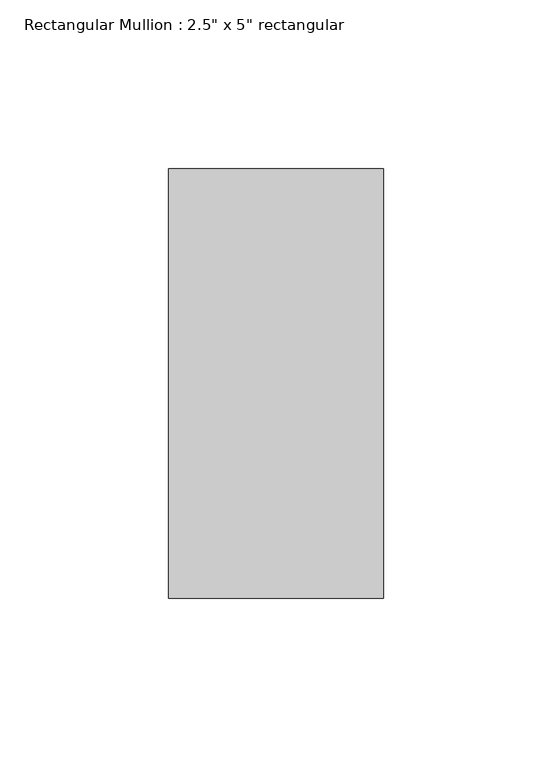
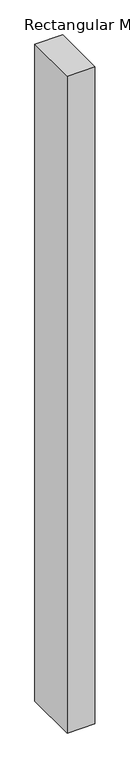
"""IFC4 building model written with IfcOpenShell, lengths in millimetres: member geometry."""

from ifc_helpers import new_model, si_unit, frame, origin, place, context, project, spatial, polyline, outline, extrude, source, transform, mapped, element, save


def member_0b703233(model_context):
    return source(origin(), model_context, "Body", "SweptSolid", [
        extrude(outline(polyline([(31.75, 63.5), (31.75, -63.5), (-31.75, -63.5), (-31.75, 63.5), (31.75, 63.5)])), frame((0.0, 0.0, -1586.2856263), z_axis=(0.0, 0.0, 1.0), x_axis=(1.0, 0.0, 0.0)), (0.0, 0.0, 1.0), 1586.2856263),
    ])


if __name__ == "__main__":
    model = new_model("IFC4")
    model_context = context("Model", 3, world=origin())
    ifc_project = project(units=[si_unit("LENGTHUNIT", "METRE", prefix="MILLI")], contexts=[model_context])
    site = spatial("IfcSite", under=ifc_project)
    building = spatial("IfcBuilding", under=site)
    placement = place(None, origin())
    member_shape = member_0b703233(model_context)
    element("IfcMember", 1, ObjectType="Rectangular Mullion : 2.5\" x 5\" rectangular", at=placement, inside=building, context=model_context, shape_type="MappedRepresentation", body=[
        mapped(member_shape, transform((0.0, 0.0, 0.0), x_axis=(1.0, 0.0, 0.0), y_axis=(0.0, 1.0, 0.0), z_axis=(0.0, 0.0, 1.0))),
    ])
    save(model, "model.ifc")

# Revit data of these elements
# Type "Rectangular Mullion : 2.5\" x 5\" rectangular"
#   built-in parameter 1007304 = 0.416667 (stored number, unit not read)
#   built-in parameter 1007301 = 0.104167 (stored number, unit not read)
#   built-in parameter 1007300 = 0.104167 (stored number, unit not read)
# Element 1 (IfcMember, "Rectangular Mullion : 2.5\" x 5\" rectangular")
#   Materials on its faces: "Aluminum"
# Materials
#   "Aluminum": class "Metal", colour RGB 247 247 247, transparency 0, Description = "Aluminum 6061", Cost = 0
